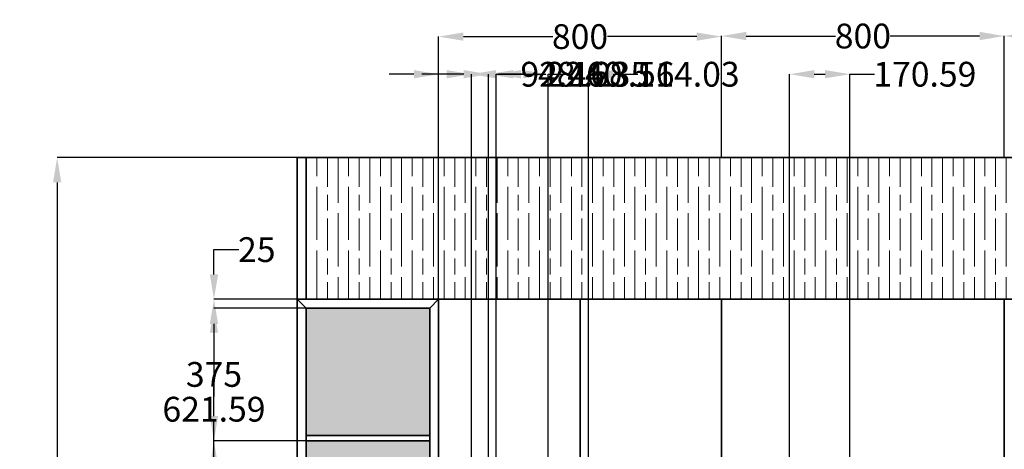
# Model space of a CAD drawing. Units: inches. Extents: x 600 to 5582, y -464 to 3142.
# Tile 6 of 9: x 600 to 3385, y 1928 to 3142. Entities that reach past the tile are written whole.
import ezdxf

# ---------------------------------------------------------------- set-up
doc = ezdxf.new("R2010")
doc.units = ezdxf.units.IN
doc.header["$MEASUREMENT"] = 0
for name, color, linetype, lineweight in [('A-ANNO-DIMS', 2, 'Continuous', 18), ('A-ELEV', 7, 'Continuous', 35), ('A-ELEV-PATT', 252, 'Continuous', 13)]:
    doc.layers.add(name, color=color, linetype=linetype, lineweight=lineweight)
doc.styles.get("Standard").update_dxf_attribs({"font": 'arial.ttf'})
doc.dimstyles.get("Standard").update_dxf_attribs({"dimtxt": 70, "dimasz": 70, "dimexe": 0.18, "dimexo": 0.0625, "dimgap": 0.09, "dimtad": 0, "dimtih": 1, "dimtoh": 1, "dimdec": 0, "dimzin": 0, "dimdsep": 46, "dimtxsty": 'Standard', "dimcen": 0.09, "dimadec": 0, "dimazin": 0, "dimtfac": 1, "dimtdec": 0, "dimtofl": 0, "dimtmove": 0, "dimatfit": 3, "dimfxl": 1, "dimtolj": 1, "dimtzin": 0, "dimarcsym": 0})

# ---------------------------------------------------------------- blocks, each defined once
blk = doc.blocks.new('*D1')
at = {"layer": 'A-ANNO-DIMS', "color": 0, "lineweight": -2, "transparency": 16777216}
for p, q in [((1384.7, 2752.4), (705.5, 2752.4)), ((705.7, 2682.4), (705.7, 1413.3)), ((705.7, 72.4), (705.7, 1341.6)), ((1384.7, 2.4), (705.5, 2.4))]:
    blk.add_line(p, q, dxfattribs=at)
at = {"layer": 'A-ANNO-DIMS', "color": 0, "transparency": 16777216}
for points in [[(694, 2682.4), (717.3, 2682.4), (705.7, 2752.4)], [(694, 72.4), (717.3, 72.4), (705.7, 2.4)]]:
    blk.add_solid(points, dxfattribs=at)
at = {"layer": 'Defpoints', "color": 0, "transparency": 16777216}
for p in [(1384.7, 2752.4), (705.7, 2.4), (1384.7, 2.4)]:
    blk.add_point(p, dxfattribs=at)
at = {"layer": 'A-ANNO-DIMS', "color": 0, "transparency": 16777216, "insert": (705.7, 1377.4), "char_height": 70, "attachment_point": 5}
blk.add_mtext('\\A1;2750', dxfattribs=at)
blk = doc.blocks.new('*D7')
at = {"layer": 'A-ANNO-DIMS', "color": 0, "lineweight": -2, "transparency": 16777216}
for p, q in [((1784.7, 2745.2), (1784.7, 3094.4)), ((1854.7, 3094.2), (2107.4, 3094.2)), ((2514.7, 3094.2), (2262.1, 3094.2)), ((2584.7, 2752.5), (2584.7, 3094.4))]:
    blk.add_line(p, q, dxfattribs=at)
at = {"layer": 'A-ANNO-DIMS', "color": 0, "transparency": 16777216}
for points in [[(1854.7, 3105.8), (1854.7, 3082.5), (1784.7, 3094.2)], [(2514.7, 3105.8), (2514.7, 3082.5), (2584.7, 3094.2)]]:
    blk.add_solid(points, dxfattribs=at)
at = {"layer": 'Defpoints', "color": 0, "transparency": 16777216}
for p in [(2584.7, 3094.2), (1784.7, 2745.1), (2584.7, 2752.4)]:
    blk.add_point(p, dxfattribs=at)
at = {"layer": 'A-ANNO-DIMS', "color": 0, "transparency": 16777216, "insert": (2184.7, 3094.2), "char_height": 70, "attachment_point": 5}
blk.add_mtext('\\A1;800', dxfattribs=at)
blk = doc.blocks.new('*D8')
at = {"layer": 'A-ANNO-DIMS', "color": 0, "lineweight": -2, "transparency": 16777216}
for p, q in [((2584.7, 2752.5), (2584.7, 3096)), ((2654.7, 3095.8), (2907.4, 3095.8)), ((3314.7, 3095.8), (3062.1, 3095.8)), ((3384.7, 2752.5), (3384.7, 3096))]:
    blk.add_line(p, q, dxfattribs=at)
at = {"layer": 'A-ANNO-DIMS', "color": 0, "transparency": 16777216}
for points in [[(2654.7, 3107.5), (2654.7, 3084.1), (2584.7, 3095.8)], [(3314.7, 3107.5), (3314.7, 3084.1), (3384.7, 3095.8)]]:
    blk.add_solid(points, dxfattribs=at)
at = {"layer": 'Defpoints', "color": 0, "transparency": 16777216}
for p in [(3384.7, 3095.8), (2584.7, 2752.4), (3384.7, 2752.4)]:
    blk.add_point(p, dxfattribs=at)
at = {"layer": 'A-ANNO-DIMS', "color": 0, "transparency": 16777216, "insert": (2984.7, 3095.8), "char_height": 70, "attachment_point": 5}
blk.add_mtext('\\A1;800', dxfattribs=at)
blk = doc.blocks.new('*D9')
at = {"layer": 'A-ANNO-DIMS', "color": 0, "lineweight": -2, "transparency": 16777216}
for p, q in [((3384.7, 2752.5), (3384.7, 3096.1)), ((3454.7, 3095.9), (3707.4, 3095.9)), ((4114.7, 3095.9), (3862.1, 3095.9)), ((4184.7, 2752.5), (4184.7, 3096.1))]:
    blk.add_line(p, q, dxfattribs=at)
at = {"layer": 'A-ANNO-DIMS', "color": 0, "transparency": 16777216}
for points in [[(3454.7, 3107.6), (3454.7, 3084.3), (3384.7, 3095.9)], [(4114.7, 3107.6), (4114.7, 3084.3), (4184.7, 3095.9)]]:
    blk.add_solid(points, dxfattribs=at)
at = {"layer": 'Defpoints', "color": 0, "transparency": 16777216}
for p in [(4184.7, 3095.9), (3384.7, 2752.4), (4184.7, 2752.4)]:
    blk.add_point(p, dxfattribs=at)
at = {"layer": 'A-ANNO-DIMS', "color": 0, "transparency": 16777216, "insert": (3784.7, 3095.9), "char_height": 70, "attachment_point": 5}
blk.add_mtext('\\A1;800', dxfattribs=at)
blk = doc.blocks.new('*D44')
at = {"layer": 'A-ANNO-DIMS', "color": 0, "lineweight": -2, "transparency": 16777216}
for p, q in [((1409.7, 1952.4), (1149.1, 1952.4)), ((1149.2, 1882.4), (1149.2, 1788.3)), ((1149.2, 1622.4), (1149.2, 1716.6)), ((1409.7, 1552.4), (1149.1, 1552.4))]:
    blk.add_line(p, q, dxfattribs=at)
at = {"layer": 'A-ANNO-DIMS', "color": 0, "transparency": 16777216}
for points in [[(1137.6, 1882.4), (1160.9, 1882.4), (1149.2, 1952.4)], [(1137.6, 1622.4), (1160.9, 1622.4), (1149.2, 1552.4)]]:
    blk.add_solid(points, dxfattribs=at)
at = {"layer": 'Defpoints', "color": 0, "transparency": 16777216}
for p in [(1149.2, 1952.4), (1409.7, 1952.4), (1409.7, 1552.4)]:
    blk.add_point(p, dxfattribs=at)
at = {"layer": 'A-ANNO-DIMS', "color": 0, "transparency": 16777216, "insert": (1149.2, 1752.4), "char_height": 70, "attachment_point": 5}
blk.add_mtext('\\A1;400', dxfattribs=at)
blk = doc.blocks.new('*D45')
at = {"layer": 'A-ANNO-DIMS', "color": 0, "lineweight": -2, "transparency": 16777216}
for p, q in [((1409.7, 2327.4), (1149.1, 2327.4)), ((1149.2, 2257.4), (1149.2, 2175.8)), ((1149.2, 2022.4), (1149.2, 2104.1)), ((1409.7, 1952.4), (1149.1, 1952.4))]:
    blk.add_line(p, q, dxfattribs=at)
at = {"layer": 'A-ANNO-DIMS', "color": 0, "transparency": 16777216}
for points in [[(1137.6, 2257.4), (1160.9, 2257.4), (1149.2, 2327.4)], [(1137.6, 2022.4), (1160.9, 2022.4), (1149.2, 1952.4)]]:
    blk.add_solid(points, dxfattribs=at)
at = {"layer": 'Defpoints', "color": 0, "transparency": 16777216}
for p in [(1149.2, 2327.4), (1409.7, 2327.4), (1409.7, 1952.4)]:
    blk.add_point(p, dxfattribs=at)
at = {"layer": 'A-ANNO-DIMS', "color": 0, "transparency": 16777216, "insert": (1149.2, 2139.9), "char_height": 70, "attachment_point": 5}
blk.add_mtext('\\A1;375', dxfattribs=at)
blk = doc.blocks.new('*D46')
at = {"layer": 'A-ANNO-DIMS', "color": 0, "lineweight": -2, "transparency": 16777216}
for p, q in [((1149.2, 2422.4), (1149.2, 2492.4)), ((1149.2, 2492.4), (1219.2, 2492.4)), ((1384.7, 2352.4), (1149.1, 2352.4)), ((1409.7, 2327.4), (1149.1, 2327.4)), ((1149.2, 2257.4), (1149.2, 2187.4))]:
    blk.add_line(p, q, dxfattribs=at)
at = {"layer": 'A-ANNO-DIMS', "color": 0, "transparency": 16777216}
for points in [[(1137.6, 2422.4), (1160.9, 2422.4), (1149.2, 2352.4)], [(1137.6, 2257.4), (1160.9, 2257.4), (1149.2, 2327.4)]]:
    blk.add_solid(points, dxfattribs=at)
at = {"layer": 'Defpoints', "color": 0, "transparency": 16777216}
for p in [(1149.2, 2352.4), (1384.7, 2352.4), (1409.7, 2327.4)]:
    blk.add_point(p, dxfattribs=at)
at = {"layer": 'A-ANNO-DIMS', "color": 0, "transparency": 16777216, "insert": (1270.3, 2492.4), "char_height": 70, "attachment_point": 5}
blk.add_mtext('\\A1;25', dxfattribs=at)
blk = doc.blocks.new('*D63')
at = {"layer": 'A-ANNO-DIMS', "color": 0, "lineweight": -2, "transparency": 16777216}
for p, q in [((2584.7, 2352.4), (1149.1, 2352.4)), ((1149.2, 2282.4), (1149.2, 2077.5)), ((1149.2, 1800.8), (1149.2, 2005.8)), ((2584.7, 1730.8), (1149.1, 1730.8))]:
    blk.add_line(p, q, dxfattribs=at)
at = {"layer": 'A-ANNO-DIMS', "color": 0, "transparency": 16777216}
for points in [[(1137.6, 2282.4), (1160.9, 2282.4), (1149.2, 2352.4)], [(1137.6, 1800.8), (1160.9, 1800.8), (1149.2, 1730.8)]]:
    blk.add_solid(points, dxfattribs=at)
at = {"layer": 'Defpoints', "color": 0, "transparency": 16777216}
for p in [(1149.2, 2352.4), (2584.7, 2352.4), (2584.7, 1730.8)]:
    blk.add_point(p, dxfattribs=at)
at = {"layer": 'A-ANNO-DIMS', "color": 0, "transparency": 16777216, "insert": (1149.2, 2041.6), "char_height": 70, "attachment_point": 5}
blk.add_mtext('\\A1;621.59', dxfattribs=at)
blk = doc.blocks.new('*D65')
at = {"layer": 'A-ANNO-DIMS', "color": 0, "lineweight": -2, "transparency": 16777216}
for p, q in [((1784.7, 2352.4), (1784.7, -233.3)), ((2184.7, 2352.4), (2184.7, -233.3)), ((1714.7, -233.1), (1644.7, -233.1)), ((2254.7, -233.1), (2324.7, -233.1))]:
    blk.add_line(p, q, dxfattribs=at)
at = {"layer": 'A-ANNO-DIMS', "color": 0, "transparency": 16777216}
for points in [[(1714.7, -221.4), (1714.7, -244.7), (1784.7, -233.1)], [(2254.7, -221.4), (2254.7, -244.7), (2184.7, -233.1)]]:
    blk.add_solid(points, dxfattribs=at)
at = {"layer": 'Defpoints', "color": 0, "transparency": 16777216}
for p in [(1784.7, 2352.4), (2184.7, 2352.4), (2184.7, -233.1)]:
    blk.add_point(p, dxfattribs=at)
at = {"layer": 'A-ANNO-DIMS', "color": 0, "transparency": 16777216, "insert": (1984.7, -233.1), "char_height": 70, "attachment_point": 5}
blk.add_mtext('\\A1;400.00', dxfattribs=at)
blk = doc.blocks.new('*D71')
at = {"layer": 'A-ANNO-DIMS', "color": 0, "lineweight": -2, "transparency": 16777216}
for p, q in [((2777.3, 1234.1), (2777.3, 2988.1)), ((2847.3, 2987.9), (2877.8, 2987.9)), ((2947.8, 1234.1), (2947.8, 2988.1)), ((2947.8, 2987.9), (3017.8, 2987.9))]:
    blk.add_line(p, q, dxfattribs=at)
at = {"layer": 'A-ANNO-DIMS', "color": 0, "transparency": 16777216}
for points in [[(2847.3, 2999.6), (2847.3, 2976.3), (2777.3, 2987.9)], [(2877.8, 2999.6), (2877.8, 2976.3), (2947.8, 2987.9)]]:
    blk.add_solid(points, dxfattribs=at)
at = {"layer": 'Defpoints', "color": 0, "transparency": 16777216}
for p in [(2947.8, 2987.9), (2777.3, 1234), (2947.8, 1234)]:
    blk.add_point(p, dxfattribs=at)
at = {"layer": 'A-ANNO-DIMS', "color": 0, "transparency": 16777216, "insert": (3160, 2987.9), "char_height": 70, "attachment_point": 5}
blk.add_mtext('\\A1;170.59', dxfattribs=at)
blk = doc.blocks.new('*D79')
at = {"layer": 'A-ANNO-DIMS', "color": 0, "lineweight": -2, "transparency": 16777216}
for p, q in [((1855.7, 2987.9), (1785.7, 2987.9)), ((1925.7, 1126.2), (1925.7, 2988.1)), ((1947.9, 1126.2), (1947.9, 2988.1)), ((2017.9, 2987.9), (2087.9, 2987.9))]:
    blk.add_line(p, q, dxfattribs=at)
at = {"layer": 'A-ANNO-DIMS', "color": 0, "transparency": 16777216}
for points in [[(1855.7, 2999.6), (1855.7, 2976.3), (1925.7, 2987.9)], [(2017.9, 2999.6), (2017.9, 2976.3), (1947.9, 2987.9)]]:
    blk.add_solid(points, dxfattribs=at)
at = {"layer": 'Defpoints', "color": 0, "transparency": 16777216}
for p in [(1947.9, 2987.9), (1925.7, 1126.1), (1947.9, 1126.1)]:
    blk.add_point(p, dxfattribs=at)
at = {"layer": 'A-ANNO-DIMS', "color": 0, "transparency": 16777216, "insert": (2234.2, 2987.9), "char_height": 70, "attachment_point": 5}
blk.add_mtext('\\A1;22.235', dxfattribs=at)
blk = doc.blocks.new('*D86')
at = {"layer": 'A-ANNO-DIMS', "color": 0, "lineweight": -2, "transparency": 16777216}
for p, q in [((1714.7, 2987.9), (1644.7, 2987.9)), ((1784.7, 1602.5), (1784.7, 2988.1)), ((1877.2, 1562.7), (1877.2, 2988.1)), ((1947.2, 2987.9), (2017.2, 2987.9))]:
    blk.add_line(p, q, dxfattribs=at)
at = {"layer": 'A-ANNO-DIMS', "color": 0, "transparency": 16777216}
for points in [[(1714.7, 2999.6), (1714.7, 2976.3), (1784.7, 2987.9)], [(1947.2, 2999.6), (1947.2, 2976.3), (1877.2, 2987.9)]]:
    blk.add_solid(points, dxfattribs=at)
at = {"layer": 'Defpoints', "color": 0, "transparency": 16777216}
for p in [(1877.2, 2987.9), (1784.7, 1602.4), (1877.2, 1562.6)]:
    blk.add_point(p, dxfattribs=at)
at = {"layer": 'A-ANNO-DIMS', "color": 0, "transparency": 16777216, "insert": (2135.4, 2987.9), "char_height": 70, "attachment_point": 5}
blk.add_mtext('\\A1;92.46', dxfattribs=at)
blk = doc.blocks.new('*D89')
at = {"layer": 'A-ANNO-DIMS', "color": 0, "lineweight": -2, "transparency": 16777216}
for p, q in [((1807.2, 2987.9), (1737.2, 2987.9)), ((1877.2, 1533.5), (1877.2, 2988.1)), ((1925.6, 1533.5), (1925.6, 2988.1)), ((1995.6, 2987.9), (2065.6, 2987.9))]:
    blk.add_line(p, q, dxfattribs=at)
at = {"layer": 'A-ANNO-DIMS', "color": 0, "transparency": 16777216}
for points in [[(1807.2, 2999.6), (1807.2, 2976.3), (1877.2, 2987.9)], [(1995.6, 2999.6), (1995.6, 2976.3), (1925.6, 2987.9)]]:
    blk.add_solid(points, dxfattribs=at)
at = {"layer": 'Defpoints', "color": 0, "transparency": 16777216}
for p in [(1925.6, 2987.9), (1877.2, 1533.5), (1925.6, 1533.5)]:
    blk.add_point(p, dxfattribs=at)
at = {"layer": 'A-ANNO-DIMS', "color": 0, "transparency": 16777216, "insert": (2185.1, 2987.9), "char_height": 70, "attachment_point": 5}
blk.add_mtext('\\A1;48.40', dxfattribs=at)
blk = doc.blocks.new('*D90')
at = {"layer": 'A-ANNO-DIMS', "color": 0, "lineweight": -2, "transparency": 16777216}
for p, q in [((1925.6, 1533.5), (1925.6, 2988.1)), ((1995.6, 2987.9), (2024.2, 2987.9)), ((2094.2, 1533.5), (2094.2, 2988.1)), ((2094.2, 2987.9), (2164.2, 2987.9))]:
    blk.add_line(p, q, dxfattribs=at)
at = {"layer": 'A-ANNO-DIMS', "color": 0, "transparency": 16777216}
for points in [[(1995.6, 2999.6), (1995.6, 2976.3), (1925.6, 2987.9)], [(2024.2, 2999.6), (2024.2, 2976.3), (2094.2, 2987.9)]]:
    blk.add_solid(points, dxfattribs=at)
at = {"layer": 'Defpoints', "color": 0, "transparency": 16777216}
for p in [(2094.2, 2987.9), (1925.6, 1533.5), (2094.2, 1533.5)]:
    blk.add_point(p, dxfattribs=at)
at = {"layer": 'A-ANNO-DIMS', "color": 0, "transparency": 16777216, "insert": (2306.2, 2987.9), "char_height": 70, "attachment_point": 5}
blk.add_mtext('\\A1;168.56', dxfattribs=at)
blk = doc.blocks.new('*D91')
at = {"layer": 'A-ANNO-DIMS', "color": 0, "lineweight": -2, "transparency": 16777216}
for p, q in [((2024.2, 2987.9), (1954.2, 2987.9)), ((2094.2, 1533.5), (2094.2, 2988.1)), ((2208.2, 1533.5), (2208.2, 2988.1)), ((2278.2, 2987.9), (2348.2, 2987.9))]:
    blk.add_line(p, q, dxfattribs=at)
at = {"layer": 'A-ANNO-DIMS', "color": 0, "transparency": 16777216}
for points in [[(2024.2, 2999.6), (2024.2, 2976.3), (2094.2, 2987.9)], [(2278.2, 2999.6), (2278.2, 2976.3), (2208.2, 2987.9)]]:
    blk.add_solid(points, dxfattribs=at)
at = {"layer": 'Defpoints', "color": 0, "transparency": 16777216}
for p in [(2208.2, 2987.9), (2094.2, 1533.5), (2208.2, 1533.5)]:
    blk.add_point(p, dxfattribs=at)
at = {"layer": 'A-ANNO-DIMS', "color": 0, "transparency": 16777216, "insert": (2490.3, 2987.9), "char_height": 70, "attachment_point": 5}
blk.add_mtext('\\A1;114.03', dxfattribs=at)

msp = doc.modelspace()

# ---------------------------------------------------------------- hatches: boundary and pattern name
at = {"layer": 'A-ELEV-PATT'}
h = msp.add_hatch(dxfattribs=at)
h.set_pattern_fill('GOST_WOOD', color=256, scale=15)
h.set_pattern_definition([(90, (0, 0), (90, -6e-15), [150, -30]), (90, (30, -30), (90, -6e-15), [90, -22.5, 45, -22.5]), (90, (60, -75), (90, -6e-15), [150, -30])])
h.paths.add_polyline_path([(4959.7485, 2752.4212), (1409.7485, 2752.4212), (1409.7485, 2352.4212), (1784.7485, 2352.4212), (4959.7485, 2352.4212)])
h.paths.add_polyline_path([(3384.7485, 1002.4212), (2584.7485, 1002.4212), (2584.7485, 777.4212), (3384.7485, 777.4212)])
h.paths.add_polyline_path([(3384.7485, 777.4212), (2584.7485, 777.4212), (2584.7485, 552.4212), (3384.7485, 552.4212)])
h.paths.add_polyline_path([(3384.7485, 512.4212), (2584.7485, 512.4212), (2584.7485, 102.4212), (3384.7485, 102.4212)])
h = msp.add_hatch(dxfattribs=at)
h.set_pattern_fill('CROSS', color=256, scale=100)
h.paths.add_polyline_path([(1759.7485, 2327.4212), (1409.7485, 2327.4212), (1409.7485, 1967.4212), (1759.7485, 1967.4212)])
h.paths.add_polyline_path([(1759.7485, 1952.4212), (1409.7485, 1952.4212), (1409.7485, 1567.4212), (1759.7485, 1567.4212)])
h.paths.add_polyline_path([(1759.7485, 1552.4212), (1409.7485, 1552.4212), (1409.7485, 1167.4212), (1759.7485, 1167.4212)])
h.paths.add_polyline_path([(1759.7485, 1152.4212), (1409.7485, 1152.4212), (1409.7485, 767.4212), (1759.7485, 767.4212)])
h.paths.add_polyline_path([(1759.7485, 752.4212), (1409.7485, 752.4212), (1409.7485, 367.4212), (1759.7485, 367.4212)])
h.paths.add_polyline_path([(1759.7485, 352.4212), (1409.7485, 352.4212), (1409.7485, 142.4212), (1759.7485, 142.4212)])
h.paths.add_polyline_path([(3759.7485, 1977.4212), (3409.7485, 1977.4212), (3409.7485, 1627.4212), (3759.7485, 1627.4212)])
h.paths.add_polyline_path([(3714.7508, 1954.858, -1), (3750.8891, 1954.858, -1)], flags=16)
h.paths.add_polyline_path([(3759.7485, 2327.4212), (3409.7485, 2327.4212), (3409.7485, 2002.4212), (3759.7485, 2002.4212)])
h.paths.add_polyline_path([(4159.7485, 2327.4212), (3809.7485, 2327.4212), (3809.7485, 2002.4212), (4159.7485, 2002.4212)])
h.paths.add_polyline_path([(4159.7485, 1977.4212), (3809.7485, 1977.4212), (3813.5467, 1954.858, -1), (3849.685, 1954.858, -1), (3813.5467, 1954.858), (3809.7485, 1627.4212), (4159.7485, 1627.4212)])
h.paths.add_polyline_path([(4559.7485, 2327.4212), (4184.7485, 2327.4212), (4184.7485, 2002.4212), (4559.7485, 2002.4212)])
h.paths.add_polyline_path([(4559.7485, 1977.4212), (4184.7485, 1977.4212), (4184.7485, 1627.4212), (4559.7485, 1627.4212)])
h.paths.add_polyline_path([(4517.0704, 1954.858, -1), (4553.2087, 1954.858, -1)], flags=16)
h.paths.add_polyline_path([(4959.7485, 2327.4212), (4609.7485, 2327.4212), (4609.7485, 2002.4212), (4959.7485, 2002.4212)])
h.paths.add_polyline_path([(4959.7485, 1977.4212), (4609.7485, 1977.4212), (4609.7485, 1627.4212), (4959.7485, 1627.4212)])
h.paths.add_polyline_path([(4619.5464, 1954.858, -1), (4655.6847, 1954.858, -1)], flags=16)

# ---------------------------------------------------------------- linework, layer by layer
at = {"layer": 'A-ELEV'}
for p, q in [((1409.7485, 2352.4212), (1409.7485, 2752.4212)), ((4984.7485, 2352.4212), (1384.7485, 2352.4212)), ((1409.7485, 1967.4212), (1759.7485, 1967.4212)), ((1409.7485, 1952.4212), (1759.7485, 1952.4212))]:
    msp.add_line(p, q, dxfattribs=at)
msp.add_lwpolyline([(4984.7485, 2.4212), (4984.7485, 2752.4212), (1384.7485, 2752.4212), (1384.7485, 2.4212)], close=True, dxfattribs=at)
for points in [[(1784.7485, 2.4212), (1784.7485, 2352.4212), (1384.7485, 2352.4212), (1409.7485, 2327.4212), (1759.7485, 2327.4212), (1409.7485, 2327.4212), (1409.7485, 127.4212)], [(1759.7485, 127.4212), (1759.7485, 2327.4212), (1784.7485, 2352.4212), (2184.7485, 2352.4212), (2184.7485, 1602.4212)], [(1784.7485, 1602.4212), (2584.7485, 1602.4212), (2584.7485, 2352.4212)], [(4984.7485, 1602.4212), (3384.7485, 1602.4212), (3384.7485, 2352.4212), (3784.7485, 2352.4212)]]:
    msp.add_lwpolyline(points, dxfattribs=at)

# ---------------------------------------------------------------- dimensions: what is measured, and where the dimension line sits
at = {"layer": 'A-ANNO-DIMS'}
for base, p1, p2, override, picture, middle in [((2584.7485, 3094.1821), (1784.7485, 2745.0995), (2584.7485, 2752.4212), {"dimclrd": 0, "dimclre": 0, "dimclrt": 0}, '*D7', (2184.7485, 3094.1821)), ((3384.7485, 3095.801), (2584.7485, 2752.4212), (3384.7485, 2752.4212), {"dimclrd": 0, "dimclre": 0, "dimclrt": 0}, '*D8', (2984.7485, 3095.801)), ((4184.7485, 3095.9369), (3384.7485, 2752.4212), (4184.7485, 2752.4212), {"dimclrd": 0, "dimclre": 0, "dimclrt": 0}, '*D9', (3784.7485, 3095.9369)), ((1877.2057, 2987.9212), (1784.7485, 1602.4212), (1877.2057, 1562.623), {"dimdec": 2, "dimlfac": 1, "dimrnd": 0, "dimzin": 0, "dimdsep": 46, "dimlunit": 2}, '*D86', (2135.3789, 2987.9212)), ((1925.6025, 2987.9212), (1877.2057, 1533.4874), (1925.6025, 1533.4874), {"dimdec": 2, "dimlfac": 1, "dimrnd": 0, "dimzin": 0, "dimdsep": 46, "dimlunit": 2}, '*D89', (2185.0889, 2987.9212)), ((1947.9344, 2987.9212), (1925.6996, 1126.1128), (1947.9344, 1126.1128), {"dimdec": 3, "dimlfac": 1, "dimrnd": 0, "dimzin": 0, "dimdsep": 46, "dimlunit": 2}, '*D79', (2234.1841, 2987.9212)), ((2094.1593, 2987.9212), (1925.6025, 1533.4874), (2094.1593, 1533.4874), {"dimdec": 2, "dimlfac": 1, "dimrnd": 0, "dimzin": 0, "dimdsep": 46, "dimlunit": 2}, '*D90', (2306.2308, 2987.9212)), ((2208.185, 2987.9212), (2094.1593, 1533.4874), (2208.185, 1533.4874), {"dimdec": 2, "dimlfac": 1, "dimrnd": 0, "dimzin": 0, "dimdsep": 46, "dimlunit": 2}, '*D91', (2490.2805, 2987.9212)), ((2947.8448, 2987.9212), (2777.2556, 1234.0488), (2947.8448, 1234.0488), {"dimdec": 2, "dimlfac": 1, "dimrnd": 0, "dimzin": 0, "dimdsep": 46, "dimlunit": 2}, '*D71', (3160.0119, 2987.9212)), ((2184.7485, -233.0788), (1784.7485, 2352.4212), (2184.7485, 2352.4212), {"dimdec": 2, "dimlfac": 1, "dimrnd": 0, "dimzin": 0, "dimdsep": 46, "dimlunit": 2}, '*D65', (1984.7485, -233.0788))]:
    dim = msp.add_linear_dim(base=base, p1=p1, p2=p2, dimstyle='Standard', override=override, dxfattribs=at)
    dim.commit()
    dim.dimension.update_dxf_attribs({"geometry": picture, "text_midpoint": middle})
for base, p1, p2, override, picture, middle in [((705.6833, 2.4212), (1384.7485, 2752.4212), (1384.7485, 2.4212), {"dimclrd": 0, "dimclre": 0, "dimclrt": 0}, '*D1', (705.6833, 1377.4212)), ((1149.2485, 2352.4212), (1409.7485, 2327.4212), (1384.7485, 2352.4212), {"dimdec": 0, "dimlfac": 1, "dimrnd": 0, "dimzin": 0, "dimdsep": 46, "dimlunit": 2}, '*D46', (1270.3344, 2492.4212)), ((1149.2485, 2352.4212), (2584.7485, 1730.8271), (2584.7485, 2352.4212), {"dimdec": 2, "dimlfac": 1, "dimrnd": 0, "dimzin": 0, "dimdsep": 46, "dimlunit": 2}, '*D63', (1149.2485, 2041.6241)), ((1149.2485, 2327.4212), (1409.7485, 1952.4212), (1409.7485, 2327.4212), {"dimdec": 0, "dimlfac": 1, "dimrnd": 0, "dimzin": 0, "dimdsep": 46, "dimlunit": 2}, '*D45', (1149.2485, 2139.9212)), ((1149.2485, 1952.4212), (1409.7485, 1552.4212), (1409.7485, 1952.4212), {"dimdec": 0, "dimlfac": 1, "dimrnd": 0, "dimzin": 0, "dimdsep": 46, "dimlunit": 2}, '*D44', (1149.2485, 1752.4212))]:
    dim = msp.add_linear_dim(base=base, p1=p1, p2=p2, angle=90, dimstyle='Standard', override=override, dxfattribs=at)
    dim.commit()
    dim.dimension.update_dxf_attribs({"geometry": picture, "text_midpoint": middle})

doc.saveas('drawing.dxf')
